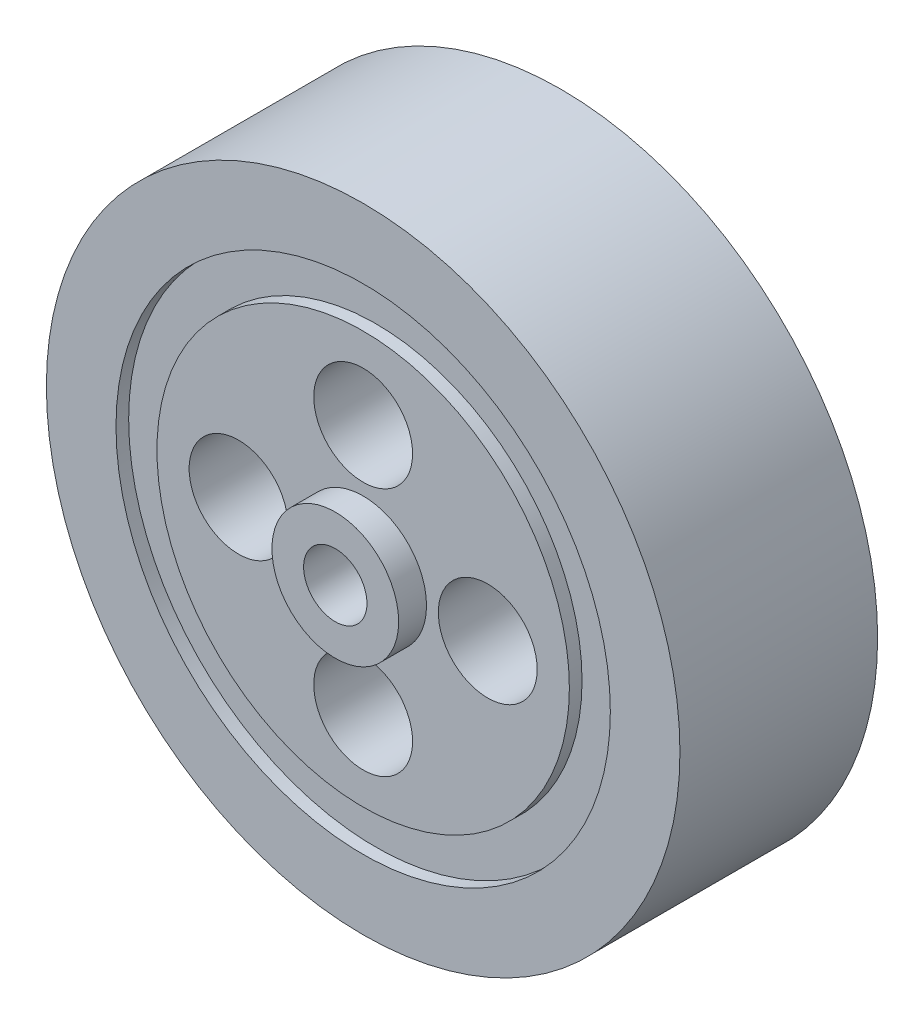
ISO-10303-21;
HEADER;
FILE_DESCRIPTION(('STEP AP214'),'2;1');
FILE_NAME('part.step','',(''),(''),'','','');
FILE_SCHEMA(('AUTOMOTIVE_DESIGN { 1 0 10303 214 1 1 1 1 }'));
ENDSEC;
DATA;
#1=APPLICATION_CONTEXT('core data for automotive mechanical design processes');
#2=APPLICATION_PROTOCOL_DEFINITION('international standard','automotive_design',2000,#1);
#3=PRODUCT_CONTEXT('',#1,'mechanical');
#4=PRODUCT('Part','Part','',(#3));
#5=PRODUCT_RELATED_PRODUCT_CATEGORY('part','',(#4));
#6=PRODUCT_DEFINITION_FORMATION('','',#4);
#7=PRODUCT_DEFINITION_CONTEXT('part definition',#1,'design');
#8=PRODUCT_DEFINITION('design','',#6,#7);
#9=PRODUCT_DEFINITION_SHAPE('','',#8);
#10=(LENGTH_UNIT() NAMED_UNIT(*) SI_UNIT(.MILLI.,.METRE.));
#11=(NAMED_UNIT(*) PLANE_ANGLE_UNIT() SI_UNIT($,.RADIAN.));
#12=(NAMED_UNIT(*) SI_UNIT($,.STERADIAN.) SOLID_ANGLE_UNIT());
#13=UNCERTAINTY_MEASURE_WITH_UNIT(LENGTH_MEASURE(1.E-05),#10,'distance_accuracy_value','');
#14=(GEOMETRIC_REPRESENTATION_CONTEXT(3) GLOBAL_UNCERTAINTY_ASSIGNED_CONTEXT((#13)) GLOBAL_UNIT_ASSIGNED_CONTEXT((#10,
#11,#12)) REPRESENTATION_CONTEXT('',''));
#15=CARTESIAN_POINT('',(0.,0.,0.));
#16=DIRECTION('',(0.,0.,1.));
#17=DIRECTION('',(1.,0.,0.));
#18=AXIS2_PLACEMENT_3D('',#15,#16,#17);
#19=CARTESIAN_POINT('',(0.,0.,-78.));
#20=DIRECTION('',(0.,0.,1.));
#21=DIRECTION('',(1.,0.,0.));
#22=AXIS2_PLACEMENT_3D('',#19,#20,#21);
#23=CYLINDRICAL_SURFACE('',#22,125.);
#24=CARTESIAN_POINT('',(0.,0.,-78.));
#25=DIRECTION('',(0.,0.,1.));
#26=DIRECTION('',(1.,0.,0.));
#27=AXIS2_PLACEMENT_3D('',#24,#25,#26);
#28=CIRCLE('',#27,125.);
#29=CARTESIAN_POINT('',(125.,0.,-78.));
#30=VERTEX_POINT('',#29);
#31=EDGE_CURVE('E10',#30,#30,#28,.T.);
#32=ORIENTED_EDGE('',*,*,#31,.T.);
#33=EDGE_LOOP('',(#32));
#34=FACE_BOUND('',#33,.T.);
#35=CARTESIAN_POINT('',(0.,0.,0.));
#36=DIRECTION('',(0.,0.,1.));
#37=DIRECTION('',(1.,0.,0.));
#38=AXIS2_PLACEMENT_3D('',#35,#36,#37);
#39=CIRCLE('',#38,125.);
#40=CARTESIAN_POINT('',(125.,0.,0.));
#41=VERTEX_POINT('',#40);
#42=EDGE_CURVE('E42',#41,#41,#39,.T.);
#43=ORIENTED_EDGE('',*,*,#42,.F.);
#44=EDGE_LOOP('',(#43));
#45=FACE_BOUND('',#44,.T.);
#46=ADVANCED_FACE('F40',(#34,#45),#23,.T.);
#47=CARTESIAN_POINT('',(0.,0.,-78.));
#48=DIRECTION('',(0.,0.,1.));
#49=DIRECTION('',(1.,0.,0.));
#50=AXIS2_PLACEMENT_3D('',#47,#48,#49);
#51=PLANE('',#50);
#52=CARTESIAN_POINT('',(0.,0.,-78.));
#53=DIRECTION('',(0.,0.,1.));
#54=DIRECTION('',(1.,0.,0.));
#55=AXIS2_PLACEMENT_3D('',#52,#53,#54);
#56=CIRCLE('',#55,12.5);
#57=CARTESIAN_POINT('',(12.5,0.,-78.));
#58=VERTEX_POINT('',#57);
#59=EDGE_CURVE('E95',#58,#58,#56,.T.);
#60=ORIENTED_EDGE('',*,*,#59,.T.);
#61=EDGE_LOOP('',(#60));
#62=FACE_BOUND('',#61,.T.);
#63=CARTESIAN_POINT('',(-49.1626298628825,0.,-78.));
#64=DIRECTION('',(0.,0.,1.));
#65=DIRECTION('',(1.,0.,0.));
#66=AXIS2_PLACEMENT_3D('',#63,#64,#65);
#67=CIRCLE('',#66,19.5);
#68=CARTESIAN_POINT('',(-29.6626298628826,0.,-78.));
#69=VERTEX_POINT('',#68);
#70=EDGE_CURVE('E76',#69,#69,#67,.T.);
#71=ORIENTED_EDGE('',*,*,#70,.T.);
#72=EDGE_LOOP('',(#71));
#73=FACE_BOUND('',#72,.T.);
#74=CARTESIAN_POINT('',(0.,-49.1626298628825,-78.));
#75=DIRECTION('',(0.,0.,1.));
#76=DIRECTION('',(1.,0.,0.));
#77=AXIS2_PLACEMENT_3D('',#74,#75,#76);
#78=CIRCLE('',#77,19.5);
#79=CARTESIAN_POINT('',(19.5,-49.1626298628825,-78.));
#80=VERTEX_POINT('',#79);
#81=EDGE_CURVE('E75',#80,#80,#78,.T.);
#82=ORIENTED_EDGE('',*,*,#81,.T.);
#83=EDGE_LOOP('',(#82));
#84=FACE_BOUND('',#83,.T.);
#85=CARTESIAN_POINT('',(49.1626298628825,0.,-78.));
#86=DIRECTION('',(0.,0.,1.));
#87=DIRECTION('',(1.,0.,0.));
#88=AXIS2_PLACEMENT_3D('',#85,#86,#87);
#89=CIRCLE('',#88,19.5);
#90=CARTESIAN_POINT('',(68.6626298628825,0.,-78.));
#91=VERTEX_POINT('',#90);
#92=EDGE_CURVE('E68',#91,#91,#89,.T.);
#93=ORIENTED_EDGE('',*,*,#92,.T.);
#94=EDGE_LOOP('',(#93));
#95=FACE_BOUND('',#94,.T.);
#96=CARTESIAN_POINT('',(0.,49.1626298628825,-78.));
#97=DIRECTION('',(0.,0.,1.));
#98=DIRECTION('',(1.,0.,0.));
#99=AXIS2_PLACEMENT_3D('',#96,#97,#98);
#100=CIRCLE('',#99,19.5);
#101=CARTESIAN_POINT('',(19.5,49.1626298628825,-78.));
#102=VERTEX_POINT('',#101);
#103=EDGE_CURVE('E58',#102,#102,#100,.T.);
#104=ORIENTED_EDGE('',*,*,#103,.T.);
#105=EDGE_LOOP('',(#104));
#106=FACE_BOUND('',#105,.T.);
#107=ORIENTED_EDGE('',*,*,#31,.F.);
#108=EDGE_LOOP('',(#107));
#109=FACE_BOUND('',#108,.T.);
#110=ADVANCED_FACE('F98',(#62,#73,#84,#95,#106,#109),#51,.F.);
#111=CARTESIAN_POINT('',(0.,0.,0.));
#112=DIRECTION('',(0.,0.,1.));
#113=DIRECTION('',(1.,0.,0.));
#114=AXIS2_PLACEMENT_3D('',#111,#112,#113);
#115=PLANE('',#114);
#116=CARTESIAN_POINT('',(0.,0.,0.));
#117=DIRECTION('',(0.,0.,1.));
#118=DIRECTION('',(1.,0.,0.));
#119=AXIS2_PLACEMENT_3D('',#116,#117,#118);
#120=CIRCLE('',#119,97.5334042252802);
#121=CARTESIAN_POINT('',(97.5334042252802,0.,0.));
#122=VERTEX_POINT('',#121);
#123=EDGE_CURVE('E51',#122,#122,#120,.T.);
#124=ORIENTED_EDGE('',*,*,#123,.F.);
#125=EDGE_LOOP('',(#124));
#126=FACE_BOUND('',#125,.T.);
#127=ORIENTED_EDGE('',*,*,#42,.T.);
#128=EDGE_LOOP('',(#127));
#129=FACE_BOUND('',#128,.T.);
#130=ADVANCED_FACE('F116',(#126,#129),#115,.T.);
#131=CARTESIAN_POINT('',(0.,0.,-5.));
#132=DIRECTION('',(0.,0.,1.));
#133=DIRECTION('',(1.,0.,0.));
#134=AXIS2_PLACEMENT_3D('',#131,#132,#133);
#135=CYLINDRICAL_SURFACE('',#134,97.5334042252802);
#136=CARTESIAN_POINT('',(0.,0.,-5.));
#137=DIRECTION('',(0.,0.,1.));
#138=DIRECTION('',(1.,0.,0.));
#139=AXIS2_PLACEMENT_3D('',#136,#137,#138);
#140=CIRCLE('',#139,97.5334042252802);
#141=CARTESIAN_POINT('',(97.5334042252802,0.,-5.));
#142=VERTEX_POINT('',#141);
#143=EDGE_CURVE('E47',#142,#142,#140,.T.);
#144=ORIENTED_EDGE('',*,*,#143,.F.);
#145=EDGE_LOOP('',(#144));
#146=FACE_BOUND('',#145,.T.);
#147=ORIENTED_EDGE('',*,*,#123,.T.);
#148=EDGE_LOOP('',(#147));
#149=FACE_BOUND('',#148,.T.);
#150=ADVANCED_FACE('F122',(#146,#149),#135,.F.);
#151=CARTESIAN_POINT('',(0.,0.,-5.));
#152=DIRECTION('',(0.,0.,1.));
#153=DIRECTION('',(1.,0.,0.));
#154=AXIS2_PLACEMENT_3D('',#151,#152,#153);
#155=PLANE('',#154);
#156=CARTESIAN_POINT('',(0.,0.,-5.));
#157=DIRECTION('',(0.,0.,1.));
#158=DIRECTION('',(1.,0.,0.));
#159=AXIS2_PLACEMENT_3D('',#156,#157,#158);
#160=CIRCLE('',#159,81.3671489250452);
#161=CARTESIAN_POINT('',(81.3671489250452,0.,-5.));
#162=VERTEX_POINT('',#161);
#163=EDGE_CURVE('E53',#162,#162,#160,.T.);
#164=ORIENTED_EDGE('',*,*,#163,.F.);
#165=EDGE_LOOP('',(#164));
#166=FACE_BOUND('',#165,.T.);
#167=ORIENTED_EDGE('',*,*,#143,.T.);
#168=EDGE_LOOP('',(#167));
#169=FACE_BOUND('',#168,.T.);
#170=ADVANCED_FACE('F130',(#166,#169),#155,.T.);
#171=CARTESIAN_POINT('',(0.,0.,-5.));
#172=DIRECTION('',(0.,0.,1.));
#173=DIRECTION('',(1.,0.,0.));
#174=AXIS2_PLACEMENT_3D('',#171,#172,#173);
#175=CYLINDRICAL_SURFACE('',#174,81.3671489250452);
#176=ORIENTED_EDGE('',*,*,#163,.T.);
#177=EDGE_LOOP('',(#176));
#178=FACE_BOUND('',#177,.T.);
#179=CARTESIAN_POINT('',(0.,0.,0.));
#180=DIRECTION('',(0.,0.,1.));
#181=DIRECTION('',(1.,0.,0.));
#182=AXIS2_PLACEMENT_3D('',#179,#180,#181);
#183=CIRCLE('',#182,81.3671489250452);
#184=CARTESIAN_POINT('',(81.3671489250452,0.,0.));
#185=VERTEX_POINT('',#184);
#186=EDGE_CURVE('E60',#185,#185,#183,.T.);
#187=ORIENTED_EDGE('',*,*,#186,.F.);
#188=EDGE_LOOP('',(#187));
#189=FACE_BOUND('',#188,.T.);
#190=ADVANCED_FACE('F131',(#178,#189),#175,.T.);
#191=CARTESIAN_POINT('',(0.,0.,0.));
#192=DIRECTION('',(0.,0.,1.));
#193=DIRECTION('',(1.,0.,0.));
#194=AXIS2_PLACEMENT_3D('',#191,#192,#193);
#195=CIRCLE('',#194,25.);
#196=CARTESIAN_POINT('',(25.,0.,0.));
#197=VERTEX_POINT('',#196);
#198=EDGE_CURVE('E37',#197,#197,#195,.F.);
#199=ORIENTED_EDGE('',*,*,#198,.T.);
#200=EDGE_LOOP('',(#199));
#201=FACE_BOUND('',#200,.T.);
#202=CARTESIAN_POINT('',(-49.1626298628825,0.,0.));
#203=DIRECTION('',(0.,0.,1.));
#204=DIRECTION('',(1.,0.,0.));
#205=AXIS2_PLACEMENT_3D('',#202,#203,#204);
#206=CIRCLE('',#205,19.5);
#207=CARTESIAN_POINT('',(-29.6626298628826,0.,0.));
#208=VERTEX_POINT('',#207);
#209=EDGE_CURVE('E82',#208,#208,#206,.T.);
#210=ORIENTED_EDGE('',*,*,#209,.F.);
#211=EDGE_LOOP('',(#210));
#212=FACE_BOUND('',#211,.T.);
#213=CARTESIAN_POINT('',(0.,-49.1626298628825,0.));
#214=DIRECTION('',(0.,0.,1.));
#215=DIRECTION('',(1.,0.,0.));
#216=AXIS2_PLACEMENT_3D('',#213,#214,#215);
#217=CIRCLE('',#216,19.5);
#218=CARTESIAN_POINT('',(19.5,-49.1626298628825,0.));
#219=VERTEX_POINT('',#218);
#220=EDGE_CURVE('E74',#219,#219,#217,.T.);
#221=ORIENTED_EDGE('',*,*,#220,.F.);
#222=EDGE_LOOP('',(#221));
#223=FACE_BOUND('',#222,.T.);
#224=CARTESIAN_POINT('',(49.1626298628825,0.,0.));
#225=DIRECTION('',(0.,0.,1.));
#226=DIRECTION('',(1.,0.,0.));
#227=AXIS2_PLACEMENT_3D('',#224,#225,#226);
#228=CIRCLE('',#227,19.5);
#229=CARTESIAN_POINT('',(68.6626298628825,0.,0.));
#230=VERTEX_POINT('',#229);
#231=EDGE_CURVE('E67',#230,#230,#228,.T.);
#232=ORIENTED_EDGE('',*,*,#231,.F.);
#233=EDGE_LOOP('',(#232));
#234=FACE_BOUND('',#233,.T.);
#235=CARTESIAN_POINT('',(0.,49.1626298628825,0.));
#236=DIRECTION('',(0.,0.,1.));
#237=DIRECTION('',(1.,0.,0.));
#238=AXIS2_PLACEMENT_3D('',#235,#236,#237);
#239=CIRCLE('',#238,19.5);
#240=CARTESIAN_POINT('',(19.5,49.1626298628825,0.));
#241=VERTEX_POINT('',#240);
#242=EDGE_CURVE('E64',#241,#241,#239,.T.);
#243=ORIENTED_EDGE('',*,*,#242,.F.);
#244=EDGE_LOOP('',(#243));
#245=FACE_BOUND('',#244,.T.);
#246=ORIENTED_EDGE('',*,*,#186,.T.);
#247=EDGE_LOOP('',(#246));
#248=FACE_BOUND('',#247,.T.);
#249=ADVANCED_FACE('F124',(#201,#212,#223,#234,#245,#248),#115,.T.);
#250=CARTESIAN_POINT('',(0.,49.1626298628825,-78.));
#251=DIRECTION('',(0.,0.,1.));
#252=DIRECTION('',(1.,0.,0.));
#253=AXIS2_PLACEMENT_3D('',#250,#251,#252);
#254=CYLINDRICAL_SURFACE('',#253,19.5);
#255=ORIENTED_EDGE('',*,*,#103,.F.);
#256=EDGE_LOOP('',(#255));
#257=FACE_BOUND('',#256,.T.);
#258=ORIENTED_EDGE('',*,*,#242,.T.);
#259=EDGE_LOOP('',(#258));
#260=FACE_BOUND('',#259,.T.);
#261=ADVANCED_FACE('F135',(#257,#260),#254,.F.);
#262=CARTESIAN_POINT('',(49.1626298628825,0.,-78.));
#263=DIRECTION('',(0.,0.,1.));
#264=DIRECTION('',(1.,0.,0.));
#265=AXIS2_PLACEMENT_3D('',#262,#263,#264);
#266=CYLINDRICAL_SURFACE('',#265,19.5);
#267=ORIENTED_EDGE('',*,*,#92,.F.);
#268=EDGE_LOOP('',(#267));
#269=FACE_BOUND('',#268,.T.);
#270=ORIENTED_EDGE('',*,*,#231,.T.);
#271=EDGE_LOOP('',(#270));
#272=FACE_BOUND('',#271,.T.);
#273=ADVANCED_FACE('F139',(#269,#272),#266,.F.);
#274=CARTESIAN_POINT('',(0.,-49.1626298628825,-78.));
#275=DIRECTION('',(0.,0.,1.));
#276=DIRECTION('',(1.,0.,0.));
#277=AXIS2_PLACEMENT_3D('',#274,#275,#276);
#278=CYLINDRICAL_SURFACE('',#277,19.5);
#279=ORIENTED_EDGE('',*,*,#81,.F.);
#280=EDGE_LOOP('',(#279));
#281=FACE_BOUND('',#280,.T.);
#282=ORIENTED_EDGE('',*,*,#220,.T.);
#283=EDGE_LOOP('',(#282));
#284=FACE_BOUND('',#283,.T.);
#285=ADVANCED_FACE('F162',(#281,#284),#278,.F.);
#286=CARTESIAN_POINT('',(-49.1626298628825,0.,-78.));
#287=DIRECTION('',(0.,0.,1.));
#288=DIRECTION('',(1.,0.,0.));
#289=AXIS2_PLACEMENT_3D('',#286,#287,#288);
#290=CYLINDRICAL_SURFACE('',#289,19.5);
#291=ORIENTED_EDGE('',*,*,#70,.F.);
#292=EDGE_LOOP('',(#291));
#293=FACE_BOUND('',#292,.T.);
#294=ORIENTED_EDGE('',*,*,#209,.T.);
#295=EDGE_LOOP('',(#294));
#296=FACE_BOUND('',#295,.T.);
#297=ADVANCED_FACE('F166',(#293,#296),#290,.F.);
#298=CARTESIAN_POINT('',(0.,0.,11.));
#299=DIRECTION('',(0.,0.,1.));
#300=DIRECTION('',(1.,0.,0.));
#301=AXIS2_PLACEMENT_3D('',#298,#299,#300);
#302=PLANE('',#301);
#303=CARTESIAN_POINT('',(0.,0.,11.));
#304=DIRECTION('',(0.,0.,1.));
#305=DIRECTION('',(1.,0.,0.));
#306=AXIS2_PLACEMENT_3D('',#303,#304,#305);
#307=CIRCLE('',#306,25.);
#308=CARTESIAN_POINT('',(25.,0.,11.));
#309=VERTEX_POINT('',#308);
#310=EDGE_CURVE('E88',#309,#309,#307,.T.);
#311=ORIENTED_EDGE('',*,*,#310,.T.);
#312=EDGE_LOOP('',(#311));
#313=FACE_BOUND('',#312,.T.);
#314=CARTESIAN_POINT('',(0.,0.,11.));
#315=DIRECTION('',(0.,0.,1.));
#316=DIRECTION('',(1.,0.,0.));
#317=AXIS2_PLACEMENT_3D('',#314,#315,#316);
#318=CIRCLE('',#317,12.5);
#319=CARTESIAN_POINT('',(12.5,0.,11.));
#320=VERTEX_POINT('',#319);
#321=EDGE_CURVE('E87',#320,#320,#318,.T.);
#322=ORIENTED_EDGE('',*,*,#321,.F.);
#323=EDGE_LOOP('',(#322));
#324=FACE_BOUND('',#323,.T.);
#325=ADVANCED_FACE('F108',(#313,#324),#302,.T.);
#326=CARTESIAN_POINT('',(0.,0.,11.));
#327=DIRECTION('',(0.,0.,-1.));
#328=DIRECTION('',(-1.,0.,0.));
#329=AXIS2_PLACEMENT_3D('',#326,#327,#328);
#330=CYLINDRICAL_SURFACE('',#329,25.);
#331=ORIENTED_EDGE('',*,*,#198,.F.);
#332=EDGE_LOOP('',(#331));
#333=FACE_BOUND('',#332,.T.);
#334=ORIENTED_EDGE('',*,*,#310,.F.);
#335=EDGE_LOOP('',(#334));
#336=FACE_BOUND('',#335,.T.);
#337=ADVANCED_FACE('F103',(#333,#336),#330,.T.);
#338=CARTESIAN_POINT('',(0.,0.,11.));
#339=DIRECTION('',(0.,0.,-1.));
#340=DIRECTION('',(-1.,0.,0.));
#341=AXIS2_PLACEMENT_3D('',#338,#339,#340);
#342=CYLINDRICAL_SURFACE('',#341,12.5);
#343=ORIENTED_EDGE('',*,*,#321,.T.);
#344=EDGE_LOOP('',(#343));
#345=FACE_BOUND('',#344,.T.);
#346=ORIENTED_EDGE('',*,*,#59,.F.);
#347=EDGE_LOOP('',(#346));
#348=FACE_BOUND('',#347,.T.);
#349=ADVANCED_FACE('F100',(#345,#348),#342,.F.);
#350=CLOSED_SHELL('',(#46,#110,#130,#150,#170,#190,#249,#261,#273,#285,#297,#325,#337,#349));
#351=MANIFOLD_SOLID_BREP('B2',#350);
#352=ADVANCED_BREP_SHAPE_REPRESENTATION('',(#18,#351),#14);
#353=SHAPE_DEFINITION_REPRESENTATION(#9,#352);
ENDSEC;
END-ISO-10303-21;
